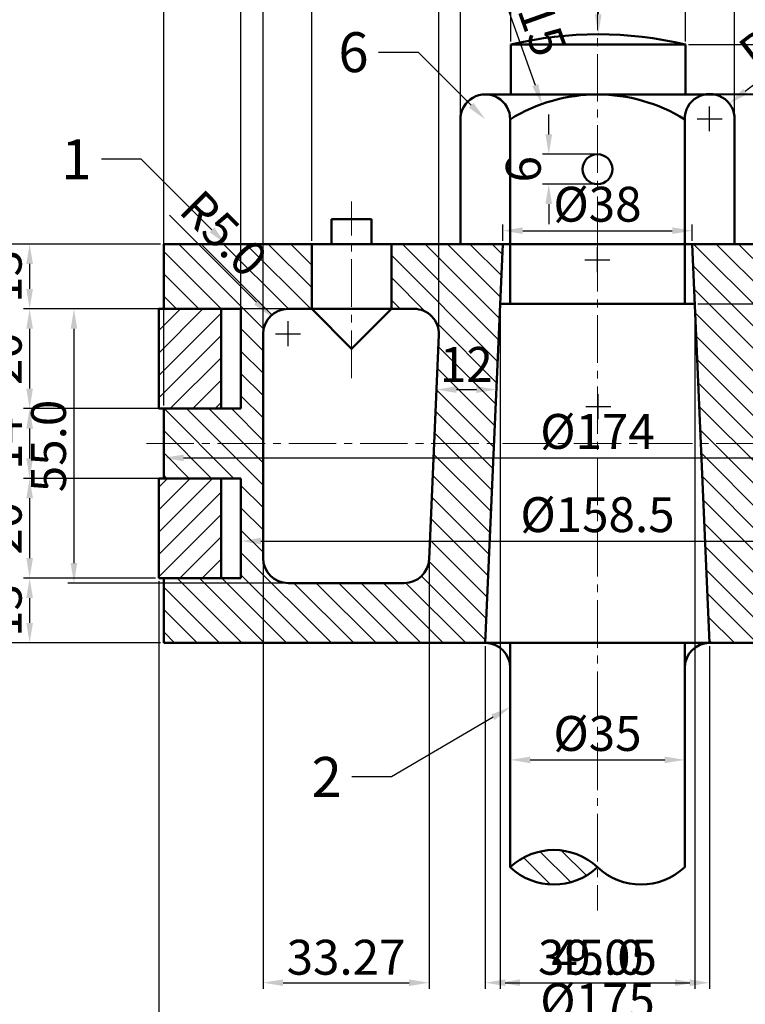
# Model space of a CAD drawing. Units: millimetres. Extents: x -21 to 693, y -570 to 295.
# Tile 4 of 7: x 107 to 253, y -4 to 193. Entities that reach past the tile are written whole.
import ezdxf
from ezdxf import colors
from ezdxf.entities.mleader import LeaderData, LeaderLine
from ezdxf.math import Vec2, Vec3

# ---------------------------------------------------------------- set-up
doc = ezdxf.new("R2010")
doc.units = ezdxf.units.MM
doc.header["$LTSCALE"] = 0.5
doc.linetypes.add('CENTER2', pattern=[28.575, 19.05, -3.175, 3.175, -3.175])
for name, color, linetype, lineweight in [('M-CNTR', 1, 'CENTER2', 18), ('M-DIMS', 2, 'Continuous', 25), ('M-HATC', 8, 'Continuous', 18), ('M-OUTL', 7, 'Continuous', 50), ('M-TEXT', 3, 'Continuous', 25)]:
    doc.layers.add(name, color=color, linetype=linetype, lineweight=lineweight)
doc.styles.get("Standard").update_dxf_attribs({"font": 'arial.ttf'})
doc.dimstyles.new('ISO-25', dxfattribs={"dimtxt": 7, "dimasz": 4, "dimexe": 1.25, "dimexo": 0.625, "dimtad": 1, "dimdec": 0, "dimtxsty": 'Standard', "dimcen": 2.5, "dimadec": 0, "dimazin": 0, "dimtfac": 1, "dimtdec": 0, "dimtofl": 0, "dimtmove": 0, "dimatfit": 3, "dimfxl": 1, "dimarcsym": 0})

# ---------------------------------------------------------------- blocks, each defined once
blk = doc.blocks.new('*U1')
at = {"layer": 'M-CNTR', "color": 0, "transparency": 16777216}
blk.add_line((0, 40), (0, -93.66), dxfattribs=at)
blk = doc.blocks.new('*U2')
at = {"layer": 'M-CNTR', "color": 0, "transparency": 16777216}
blk.add_line((90.5, 0), (-90.5, 0), dxfattribs=at)
blk = doc.blocks.new('*U3')
at = {"layer": 'M-CNTR', "color": 0, "transparency": 16777216}
blk.add_line((0, -29.38), (0, 6), dxfattribs=at)
blk = doc.blocks.new('*D5')
at = {"layer": 'Defpoints', "color": 0, "ltscale": 0.5, "transparency": 16777216}
for p in [(135.24, 81.11), (311.24, 81.11), (311.24, -8.97)]:
    blk.add_point(p, dxfattribs=at)
at = {"layer": 'M-DIMS', "color": 0, "lineweight": -2, "ltscale": 0.5, "transparency": 16777216}
for p, q in [((135.24, 80.49), (135.24, -10.22)), ((311.24, 80.49), (311.24, -10.22)), ((139.24, -8.97), (307.24, -8.97))]:
    blk.add_line(p, q, dxfattribs=at)
at = {"layer": 'M-DIMS', "color": 0, "ltscale": 0.5, "transparency": 16777216}
for points in [[(139.24, -8.31), (139.24, -9.64), (135.24, -8.97)], [(307.24, -8.31), (307.24, -9.64), (311.24, -8.97)]]:
    blk.add_solid(points, dxfattribs=at)
at = {"layer": 'M-DIMS', "color": 0, "ltscale": 0.5, "transparency": 16777216, "insert": (223.24, -4.58), "char_height": 7, "attachment_point": 5}
blk.add_mtext('%%C175', dxfattribs=at)
blk = doc.blocks.new('*D6')
at = {"layer": 'Defpoints', "color": 0, "ltscale": 0.5, "transparency": 16777216}
for p in [(136.24, 148.11), (77.7, 68.11), (136.24, 68.11)]:
    blk.add_point(p, dxfattribs=at)
at = {"layer": 'M-DIMS', "color": 0, "lineweight": -2, "ltscale": 0.5, "transparency": 16777216}
for p, q in [((135.61, 148.11), (76.45, 148.11)), ((77.7, 144.11), (77.7, 72.11)), ((135.61, 68.11), (76.45, 68.11))]:
    blk.add_line(p, q, dxfattribs=at)
at = {"layer": 'M-DIMS', "color": 0, "ltscale": 0.5, "transparency": 16777216}
for points in [[(77.04, 144.11), (78.37, 144.11), (77.7, 148.11)], [(77.04, 72.11), (78.37, 72.11), (77.7, 68.11)]]:
    blk.add_solid(points, dxfattribs=at)
at = {"layer": 'M-DIMS', "color": 0, "ltscale": 0.5, "transparency": 16777216, "insert": (73.5, 108.11), "char_height": 7, "attachment_point": 5, "rotation": 90}
blk.add_mtext('80', dxfattribs=at)
blk = doc.blocks.new('*D7')
at = {"layer": 'Defpoints', "color": 0, "ltscale": 0.5, "transparency": 16777216}
for p in [(136.24, 148.11), (109.35, 135.11), (136.24, 135.11)]:
    blk.add_point(p, dxfattribs=at)
at = {"layer": 'M-DIMS', "color": 0, "lineweight": -2, "ltscale": 0.5, "transparency": 16777216}
for p, q in [((135.61, 148.11), (108.1, 148.11)), ((109.35, 144.11), (109.35, 139.11)), ((135.61, 135.11), (108.1, 135.11))]:
    blk.add_line(p, q, dxfattribs=at)
at = {"layer": 'M-DIMS', "color": 0, "ltscale": 0.5, "transparency": 16777216}
for points in [[(108.69, 144.11), (110.02, 144.11), (109.35, 148.11)], [(108.69, 139.11), (110.02, 139.11), (109.35, 135.11)]]:
    blk.add_solid(points, dxfattribs=at)
at = {"layer": 'M-DIMS', "color": 0, "ltscale": 0.5, "transparency": 16777216, "insert": (105.15, 141.61), "char_height": 7, "attachment_point": 5, "rotation": 90}
blk.add_mtext('13', dxfattribs=at)
blk = doc.blocks.new('*D8')
at = {"layer": 'Defpoints', "color": 0, "ltscale": 0.5, "transparency": 16777216}
for p in [(135.24, 135.11), (109.35, 115.11), (136.24, 115.11)]:
    blk.add_point(p, dxfattribs=at)
at = {"layer": 'M-DIMS', "color": 0, "lineweight": -2, "ltscale": 0.5, "transparency": 16777216}
for p, q in [((134.61, 135.11), (108.1, 135.11)), ((109.35, 131.11), (109.35, 119.11)), ((135.61, 115.11), (108.1, 115.11))]:
    blk.add_line(p, q, dxfattribs=at)
at = {"layer": 'M-DIMS', "color": 0, "ltscale": 0.5, "transparency": 16777216}
for points in [[(108.69, 131.11), (110.02, 131.11), (109.35, 135.11)], [(108.69, 119.11), (110.02, 119.11), (109.35, 115.11)]]:
    blk.add_solid(points, dxfattribs=at)
at = {"layer": 'M-DIMS', "color": 0, "ltscale": 0.5, "transparency": 16777216, "insert": (105.16, 125.11), "char_height": 7, "attachment_point": 5, "rotation": 90}
blk.add_mtext('20', dxfattribs=at)
blk = doc.blocks.new('*D9')
at = {"layer": 'Defpoints', "color": 0, "ltscale": 0.5, "transparency": 16777216}
for p in [(136.24, 115.11), (109.35, 101.11), (136.24, 101.11)]:
    blk.add_point(p, dxfattribs=at)
at = {"layer": 'M-DIMS', "color": 0, "lineweight": -2, "ltscale": 0.5, "transparency": 16777216}
for p, q in [((135.61, 115.11), (108.1, 115.11)), ((109.35, 111.11), (109.35, 105.11)), ((135.61, 101.11), (108.1, 101.11))]:
    blk.add_line(p, q, dxfattribs=at)
at = {"layer": 'M-DIMS', "color": 0, "ltscale": 0.5, "transparency": 16777216}
for points in [[(108.69, 111.11), (110.02, 111.11), (109.35, 115.11)], [(108.69, 105.11), (110.02, 105.11), (109.35, 101.11)]]:
    blk.add_solid(points, dxfattribs=at)
at = {"layer": 'M-DIMS', "color": 0, "ltscale": 0.5, "transparency": 16777216, "insert": (105.21, 108.11), "char_height": 7, "attachment_point": 5, "rotation": 90}
blk.add_mtext('14', dxfattribs=at)
blk = doc.blocks.new('*D10')
at = {"layer": 'Defpoints', "color": 0, "ltscale": 0.5, "transparency": 16777216}
for p in [(136.24, 101.11), (109.35, 81.11), (135.24, 81.11)]:
    blk.add_point(p, dxfattribs=at)
at = {"layer": 'M-DIMS', "color": 0, "lineweight": -2, "ltscale": 0.5, "transparency": 16777216}
for p, q in [((135.61, 101.11), (108.1, 101.11)), ((109.35, 97.11), (109.35, 85.11)), ((134.61, 81.11), (108.1, 81.11))]:
    blk.add_line(p, q, dxfattribs=at)
at = {"layer": 'M-DIMS', "color": 0, "ltscale": 0.5, "transparency": 16777216}
for points in [[(108.69, 97.11), (110.02, 97.11), (109.35, 101.11)], [(108.69, 85.11), (110.02, 85.11), (109.35, 81.11)]]:
    blk.add_solid(points, dxfattribs=at)
at = {"layer": 'M-DIMS', "color": 0, "ltscale": 0.5, "transparency": 16777216, "insert": (105.16, 91.11), "char_height": 7, "attachment_point": 5, "rotation": 90}
blk.add_mtext('20', dxfattribs=at)
blk = doc.blocks.new('*D11')
at = {"layer": 'Defpoints', "color": 0, "ltscale": 0.5, "transparency": 16777216}
for p in [(129.36, 81.11), (109.35, 68.11), (136.24, 68.11)]:
    blk.add_point(p, dxfattribs=at)
at = {"layer": 'M-DIMS', "color": 0, "lineweight": -2, "ltscale": 0.5, "transparency": 16777216}
for p, q in [((128.74, 81.11), (108.1, 81.11)), ((109.35, 77.11), (109.35, 72.11)), ((135.61, 68.11), (108.1, 68.11))]:
    blk.add_line(p, q, dxfattribs=at)
at = {"layer": 'M-DIMS', "color": 0, "ltscale": 0.5, "transparency": 16777216}
for points in [[(108.69, 77.11), (110.02, 77.11), (109.35, 81.11)], [(108.69, 72.11), (110.02, 72.11), (109.35, 68.11)]]:
    blk.add_solid(points, dxfattribs=at)
at = {"layer": 'M-DIMS', "color": 0, "ltscale": 0.5, "transparency": 16777216, "insert": (105.15, 74.61), "char_height": 7, "attachment_point": 5, "rotation": 90}
blk.add_mtext('13', dxfattribs=at)
blk = doc.blocks.new('*D12')
at = {"layer": 'Defpoints', "color": 0, "ltscale": 0.5, "transparency": 16777216}
for p in [(190.95, 118.92), (202.96, 118.92), (202.96, 118.92)]:
    blk.add_point(p, dxfattribs=at)
at = {"layer": 'M-DIMS', "color": 0, "lineweight": -2, "ltscale": 0.5, "transparency": 16777216}
for p, q in [((190.95, 119.54), (190.95, 120.17)), ((194.95, 118.92), (198.96, 118.92)), ((202.96, 119.54), (202.96, 120.17))]:
    blk.add_line(p, q, dxfattribs=at)
at = {"layer": 'M-DIMS', "color": 0, "ltscale": 0.5, "transparency": 16777216}
for points in [[(194.95, 119.59), (194.95, 118.25), (190.95, 118.92)], [(198.96, 119.59), (198.96, 118.25), (202.96, 118.92)]]:
    blk.add_solid(points, dxfattribs=at)
at = {"layer": 'M-DIMS', "color": 0, "ltscale": 0.5, "transparency": 16777216, "insert": (196.95, 123.06), "char_height": 7, "attachment_point": 5}
blk.add_mtext('12', dxfattribs=at)
blk = doc.blocks.new('*D13')
at = {"layer": 'Defpoints', "color": 0, "ltscale": 0.5, "transparency": 16777216}
for p in [(151.74, 91.11), (294.74, 91.11), (294.74, 88.53)]:
    blk.add_point(p, dxfattribs=at)
at = {"layer": 'M-DIMS', "color": 0, "lineweight": -2, "ltscale": 0.5, "transparency": 16777216}
for p, q in [((151.74, 90.49), (151.74, 87.28)), ((294.74, 90.49), (294.74, 87.28)), ((155.74, 88.53), (290.74, 88.53))]:
    blk.add_line(p, q, dxfattribs=at)
at = {"layer": 'M-DIMS', "color": 0, "ltscale": 0.5, "transparency": 16777216}
for points in [[(155.74, 89.2), (155.74, 87.87), (151.74, 88.53)], [(290.74, 89.2), (290.74, 87.87), (294.74, 88.53)]]:
    blk.add_solid(points, dxfattribs=at)
at = {"layer": 'M-DIMS', "color": 0, "ltscale": 0.5, "transparency": 16777216, "insert": (223.24, 92.93), "char_height": 7, "attachment_point": 5}
blk.add_mtext('%%C158.5', dxfattribs=at)
blk = doc.blocks.new('*D14')
at = {"layer": 'Defpoints', "color": 0, "ltscale": 0.5, "transparency": 16777216}
for p in [(136.24, 108.11), (310.24, 108.11), (310.24, 105.22)]:
    blk.add_point(p, dxfattribs=at)
at = {"layer": 'M-DIMS', "color": 0, "lineweight": -2, "ltscale": 0.5, "transparency": 16777216}
for p, q in [((136.24, 107.49), (136.24, 103.97)), ((310.24, 107.49), (310.24, 103.97)), ((140.24, 105.22), (306.24, 105.22))]:
    blk.add_line(p, q, dxfattribs=at)
at = {"layer": 'M-DIMS', "color": 0, "ltscale": 0.5, "transparency": 16777216}
for points in [[(140.24, 105.89), (140.24, 104.55), (136.24, 105.22)], [(306.24, 105.89), (306.24, 104.55), (310.24, 105.22)]]:
    blk.add_solid(points, dxfattribs=at)
at = {"layer": 'M-DIMS', "color": 0, "ltscale": 0.5, "transparency": 16777216, "insert": (223.24, 109.62), "char_height": 7, "attachment_point": 5}
blk.add_mtext('%%C174', dxfattribs=at)
blk = doc.blocks.new('*D15')
at = {"layer": 'Defpoints', "color": 0, "ltscale": 0.5, "transparency": 16777216}
for p in [(242.24, 150.79), (204.24, 148.11), (242.24, 148.11)]:
    blk.add_point(p, dxfattribs=at)
at = {"layer": 'M-DIMS', "color": 0, "lineweight": -2, "ltscale": 0.5, "transparency": 16777216}
for p, q in [((204.24, 148.74), (204.24, 152.04)), ((208.24, 150.79), (238.24, 150.79)), ((242.24, 148.74), (242.24, 152.04))]:
    blk.add_line(p, q, dxfattribs=at)
at = {"layer": 'M-DIMS', "color": 0, "ltscale": 0.5, "transparency": 16777216}
for points in [[(208.24, 151.46), (208.24, 150.13), (204.24, 150.79)], [(238.24, 151.46), (238.24, 150.13), (242.24, 150.79)]]:
    blk.add_solid(points, dxfattribs=at)
at = {"layer": 'M-DIMS', "color": 0, "ltscale": 0.5, "transparency": 16777216, "insert": (223.24, 155.19), "char_height": 7, "attachment_point": 5}
blk.add_mtext('%%C38', dxfattribs=at)
blk = doc.blocks.new('*D16')
at = {"layer": 'Defpoints', "color": 0, "ltscale": 0.5, "transparency": 16777216}
for p in [(223.24, 166.11), (213.47, 160.11), (223.24, 160.11)]:
    blk.add_point(p, dxfattribs=at)
at = {"layer": 'M-DIMS', "color": 0, "lineweight": -2, "ltscale": 0.5, "transparency": 16777216}
for p, q in [((213.47, 170.11), (213.47, 174.11)), ((222.61, 166.11), (212.22, 166.11)), ((222.61, 160.11), (212.22, 160.11)), ((213.47, 156.11), (213.47, 152.11))]:
    blk.add_line(p, q, dxfattribs=at)
at = {"layer": 'M-DIMS', "color": 0, "ltscale": 0.5, "transparency": 16777216}
for points in [[(212.8, 170.11), (214.14, 170.11), (213.47, 166.11)], [(212.8, 156.11), (214.14, 156.11), (213.47, 160.11)]]:
    blk.add_solid(points, dxfattribs=at)
at = {"layer": 'M-DIMS', "color": 0, "ltscale": 0.5, "transparency": 16777216, "insert": (209.27, 163.11), "char_height": 7, "attachment_point": 5, "rotation": 90}
blk.add_mtext('6', dxfattribs=at)
blk = doc.blocks.new('*D17')
at = {"layer": 'Defpoints', "color": 0, "ltscale": 0.5, "transparency": 16777216}
for p in [(205.74, 45.61), (240.74, 45.61), (240.74, 44.65)]:
    blk.add_point(p, dxfattribs=at)
at = {"layer": 'M-DIMS', "color": 0, "lineweight": -2, "ltscale": 0.5, "transparency": 16777216}
for p, q in [((205.74, 44.99), (205.74, 43.4)), ((209.74, 44.65), (236.74, 44.65)), ((240.74, 44.99), (240.74, 43.4))]:
    blk.add_line(p, q, dxfattribs=at)
at = {"layer": 'M-DIMS', "color": 0, "ltscale": 0.5, "transparency": 16777216}
for points in [[(209.74, 45.31), (209.74, 43.98), (205.74, 44.65)], [(236.74, 45.31), (236.74, 43.98), (240.74, 44.65)]]:
    blk.add_solid(points, dxfattribs=at)
at = {"layer": 'M-DIMS', "color": 0, "ltscale": 0.5, "transparency": 16777216, "insert": (223.24, 49.04), "char_height": 7, "attachment_point": 5}
blk.add_mtext('%%C35', dxfattribs=at)
blk = doc.blocks.new('SCREW-PLUG')
for p, q in [((4, 21), (4, 26)), ((4, 26), (12, 26)), ((12, 26), (12, 21)), ((0, 21), (0, 8)), ((16, 21), (16, 8)), ((0, 8), (8, 0)), ((16, 8), (8, 0))]:
    blk.add_line(p, q)
blk = doc.blocks.new('*D49')
at = {"layer": 'Defpoints', "color": 0, "ltscale": 0.5, "transparency": 16777216}
for p in [(191.43, 210.86), (156.19, 130.11), (191.43, 129.89)]:
    blk.add_point(p, dxfattribs=at)
at = {"layer": 'M-DIMS', "color": 0, "lineweight": -2, "ltscale": 0.5, "transparency": 16777216}
for p, q in [((156.19, 130.74), (156.19, 212.11)), ((191.43, 130.52), (191.43, 212.11)), ((160.19, 210.86), (187.43, 210.86))]:
    blk.add_line(p, q, dxfattribs=at)
at = {"layer": 'M-DIMS', "color": 0, "ltscale": 0.5, "transparency": 16777216}
for points in [[(160.19, 211.53), (160.19, 210.2), (156.19, 210.86)], [(187.43, 211.53), (187.43, 210.2), (191.43, 210.86)]]:
    blk.add_solid(points, dxfattribs=at)
at = {"layer": 'M-DIMS', "color": 0, "ltscale": 0.5, "transparency": 16777216, "insert": (173.81, 215.07), "char_height": 7, "attachment_point": 5}
blk.add_mtext('35.24', dxfattribs=at)
blk = doc.blocks.new('*D50')
at = {"layer": 'Defpoints', "color": 0, "ltscale": 0.5, "transparency": 16777216}
for p in [(156.19, 85.11), (189.46, 84.89), (189.46, -0.04)]:
    blk.add_point(p, dxfattribs=at)
at = {"layer": 'M-DIMS', "color": 0, "lineweight": -2, "ltscale": 0.5, "transparency": 16777216}
for p, q in [((156.19, 84.49), (156.19, -1.29)), ((189.46, 84.27), (189.46, -1.29)), ((160.19, -0.04), (185.46, -0.04))]:
    blk.add_line(p, q, dxfattribs=at)
at = {"layer": 'M-DIMS', "color": 0, "ltscale": 0.5, "transparency": 16777216}
for points in [[(160.19, 0.62), (160.19, -0.71), (156.19, -0.04)], [(185.46, 0.62), (185.46, -0.71), (189.46, -0.04)]]:
    blk.add_solid(points, dxfattribs=at)
at = {"layer": 'M-DIMS', "color": 0, "ltscale": 0.5, "transparency": 16777216, "insert": (172.82, 4.16), "char_height": 7, "attachment_point": 5}
blk.add_mtext('33.27', dxfattribs=at)
blk = doc.blocks.new('*D51')
at = {"layer": 'Defpoints', "color": 0, "ltscale": 0.5, "transparency": 16777216}
for p in [(161.19, 135.11), (118.24, 80.11), (161.19, 80.11)]:
    blk.add_point(p, dxfattribs=at)
at = {"layer": 'M-DIMS', "color": 0, "lineweight": -2, "ltscale": 0.5, "transparency": 16777216}
for p, q in [((160.56, 135.11), (116.99, 135.11)), ((118.24, 131.11), (118.24, 84.11)), ((160.56, 80.11), (116.99, 80.11))]:
    blk.add_line(p, q, dxfattribs=at)
at = {"layer": 'M-DIMS', "color": 0, "ltscale": 0.5, "transparency": 16777216}
for points in [[(117.57, 131.11), (118.9, 131.11), (118.24, 135.11)], [(117.57, 84.11), (118.9, 84.11), (118.24, 80.11)]]:
    blk.add_solid(points, dxfattribs=at)
at = {"layer": 'M-DIMS', "color": 0, "ltscale": 0.5, "transparency": 16777216, "insert": (114.04, 107.61), "char_height": 7, "attachment_point": 5, "rotation": 90}
blk.add_mtext('55.0', dxfattribs=at)
blk = doc.blocks.new('*D52')
at = {"layer": 'Defpoints', "color": 0, "ltscale": 0.5, "transparency": 16777216}
for p in [(151.74, 210.86), (136.24, 115.11), (151.74, 115.11)]:
    blk.add_point(p, dxfattribs=at)
at = {"layer": 'M-DIMS', "color": 0, "lineweight": -2, "ltscale": 0.5, "transparency": 16777216}
for p, q in [((136.24, 115.74), (136.24, 212.11)), ((151.74, 115.74), (151.74, 212.11)), ((140.24, 210.86), (147.74, 210.86)), ((151.74, 210.86), (174.56, 210.86))]:
    blk.add_line(p, q, dxfattribs=at)
at = {"layer": 'M-DIMS', "color": 0, "ltscale": 0.5, "transparency": 16777216}
for points in [[(140.24, 211.53), (140.24, 210.2), (136.24, 210.86)], [(147.74, 211.53), (147.74, 210.2), (151.74, 210.86)]]:
    blk.add_solid(points, dxfattribs=at)
at = {"layer": 'M-DIMS', "color": 0, "ltscale": 0.5, "transparency": 16777216, "insert": (165.15, 215.06), "char_height": 7, "attachment_point": 5}
blk.add_mtext('15.5', dxfattribs=at)
blk = doc.blocks.new('*D53')
at = {"layer": 'Defpoints', "color": 0, "ltscale": 0.5, "transparency": 16777216}
for p in [(203.71, 136.11), (242.76, 136.11), (242.76, -0.04)]:
    blk.add_point(p, dxfattribs=at)
at = {"layer": 'M-DIMS', "color": 0, "lineweight": -2, "ltscale": 0.5, "transparency": 16777216}
for p, q in [((203.71, 135.49), (203.71, -1.29)), ((242.76, 135.49), (242.76, -1.29)), ((207.71, -0.04), (238.76, -0.04))]:
    blk.add_line(p, q, dxfattribs=at)
at = {"layer": 'M-DIMS', "color": 0, "ltscale": 0.5, "transparency": 16777216}
for points in [[(207.71, 0.62), (207.71, -0.71), (203.71, -0.04)], [(238.76, 0.62), (238.76, -0.71), (242.76, -0.04)]]:
    blk.add_solid(points, dxfattribs=at)
at = {"layer": 'M-DIMS', "color": 0, "ltscale": 0.5, "transparency": 16777216, "insert": (223.24, 4.16), "char_height": 7, "attachment_point": 5}
blk.add_mtext('39.05', dxfattribs=at)
blk = doc.blocks.new('*D54')
at = {"layer": 'Defpoints', "color": 0, "ltscale": 0.5, "transparency": 16777216}
for p in [(200.74, 68.11), (245.74, 68.11), (245.74, -0.04)]:
    blk.add_point(p, dxfattribs=at)
at = {"layer": 'M-DIMS', "color": 0, "lineweight": -2, "ltscale": 0.5, "transparency": 16777216}
for p, q in [((200.74, 67.49), (200.74, -1.29)), ((245.74, 67.49), (245.74, -1.29)), ((204.74, -0.04), (241.74, -0.04))]:
    blk.add_line(p, q, dxfattribs=at)
at = {"layer": 'M-DIMS', "color": 0, "ltscale": 0.5, "transparency": 16777216}
for points in [[(204.74, 0.62), (204.74, -0.71), (200.74, -0.04)], [(241.74, 0.62), (241.74, -0.71), (245.74, -0.04)]]:
    blk.add_solid(points, dxfattribs=at)
at = {"layer": 'M-DIMS', "color": 0, "ltscale": 0.5, "transparency": 16777216, "insert": (223.24, 4.16), "char_height": 7, "attachment_point": 5}
blk.add_mtext('45.0', dxfattribs=at)
blk = doc.blocks.new('*D55')
at = {"layer": 'Defpoints', "color": 0, "ltscale": 0.5, "transparency": 16777216}
for p in [(242.24, 148.11), (242.76, 136.11), (328.24, 136.11)]:
    blk.add_point(p, dxfattribs=at)
at = {"layer": 'M-DIMS', "color": 0, "lineweight": -2, "ltscale": 0.5, "transparency": 16777216}
for p, q in [((242.86, 148.11), (329.49, 148.11)), ((328.24, 144.11), (328.24, 140.11)), ((243.39, 136.11), (329.49, 136.11)), ((328.24, 136.11), (328.24, 113.36))]:
    blk.add_line(p, q, dxfattribs=at)
at = {"layer": 'M-DIMS', "color": 0, "ltscale": 0.5, "transparency": 16777216}
for points in [[(327.57, 144.11), (328.9, 144.11), (328.24, 148.11)], [(327.57, 140.11), (328.9, 140.11), (328.24, 136.11)]]:
    blk.add_solid(points, dxfattribs=at)
at = {"layer": 'M-DIMS', "color": 0, "ltscale": 0.5, "transparency": 16777216, "insert": (324.04, 122.74), "char_height": 7, "attachment_point": 5, "rotation": 90}
blk.add_mtext('12.0', dxfattribs=at)
blk = doc.blocks.new('*D56')
at = {"layer": 'Defpoints', "color": 0, "ltscale": 0.5, "transparency": 16777216}
for p in [(165.92, 210.86), (136.24, 148.11), (165.92, 148.11)]:
    blk.add_point(p, dxfattribs=at)
at = {"layer": 'M-DIMS', "color": 0, "lineweight": -2, "ltscale": 0.5, "transparency": 16777216}
for p, q in [((136.24, 148.74), (136.24, 212.11)), ((165.92, 148.74), (165.92, 212.11)), ((140.24, 210.86), (161.92, 210.86)), ((165.92, 210.86), (200.4, 210.86))]:
    blk.add_line(p, q, dxfattribs=at)
at = {"layer": 'M-DIMS', "color": 0, "ltscale": 0.5, "transparency": 16777216}
for points in [[(140.24, 211.53), (140.24, 210.2), (136.24, 210.86)], [(161.92, 211.53), (161.92, 210.2), (165.92, 210.86)]]:
    blk.add_solid(points, dxfattribs=at)
at = {"layer": 'M-DIMS', "color": 0, "ltscale": 0.5, "transparency": 16777216, "insert": (185.16, 215.06), "char_height": 7, "attachment_point": 5}
blk.add_mtext('29.685', dxfattribs=at)
blk = doc.blocks.new('*D61')
at = {"layer": 'Defpoints', "color": 0, "ltscale": 0.5, "transparency": 16777216}
for p in [(250.74, 210.86), (195.74, 173.12), (250.74, 173.32)]:
    blk.add_point(p, dxfattribs=at)
at = {"layer": 'M-DIMS', "color": 0, "lineweight": -2, "ltscale": 0.5, "transparency": 16777216}
for p, q in [((195.74, 173.75), (195.74, 212.11)), ((250.74, 173.95), (250.74, 212.11)), ((199.74, 210.86), (246.74, 210.86))]:
    blk.add_line(p, q, dxfattribs=at)
at = {"layer": 'M-DIMS', "color": 0, "ltscale": 0.5, "transparency": 16777216}
for points in [[(199.74, 211.53), (199.74, 210.2), (195.74, 210.86)], [(246.74, 211.53), (246.74, 210.2), (250.74, 210.86)]]:
    blk.add_solid(points, dxfattribs=at)
at = {"layer": 'M-DIMS', "color": 0, "ltscale": 0.5, "transparency": 16777216, "insert": (223.24, 215.06), "char_height": 7, "attachment_point": 5}
blk.add_mtext('55.0', dxfattribs=at)
blk = doc.blocks.new('*D62')
at = {"layer": 'Defpoints', "color": 0, "ltscale": 0.5, "transparency": 16777216}
for p in [(245.74, 178.22), (328.24, 178.22), (250.74, 148.11)]:
    blk.add_point(p, dxfattribs=at)
at = {"layer": 'M-DIMS', "color": 0, "lineweight": -2, "ltscale": 0.5, "transparency": 16777216}
for p, q in [((328.24, 178.22), (328.24, 212.58)), ((246.36, 178.22), (329.49, 178.22)), ((328.24, 152.11), (328.24, 174.22)), ((251.36, 148.11), (329.49, 148.11))]:
    blk.add_line(p, q, dxfattribs=at)
at = {"layer": 'M-DIMS', "color": 0, "ltscale": 0.5, "transparency": 16777216}
for points in [[(327.57, 174.22), (328.9, 174.22), (328.24, 178.22)], [(327.57, 152.11), (328.9, 152.11), (328.24, 148.11)]]:
    blk.add_solid(points, dxfattribs=at)
at = {"layer": 'M-DIMS', "color": 0, "ltscale": 0.5, "transparency": 16777216, "insert": (324.04, 197.4), "char_height": 7, "attachment_point": 5, "rotation": 90}
blk.add_mtext('30.105', dxfattribs=at)
blk = doc.blocks.new('*D63')
at = {"layer": 'Defpoints', "color": 0, "ltscale": 0.5, "transparency": 16777216}
for p in [(240.89, 210.86), (205.89, 188.11), (240.89, 188.11)]:
    blk.add_point(p, dxfattribs=at)
at = {"layer": 'M-DIMS', "color": 0, "lineweight": -2, "ltscale": 0.5, "transparency": 16777216}
for p, q in [((205.89, 188.74), (205.89, 212.11)), ((240.89, 188.74), (240.89, 212.11)), ((209.89, 210.86), (236.89, 210.86))]:
    blk.add_line(p, q, dxfattribs=at)
at = {"layer": 'M-DIMS', "color": 0, "ltscale": 0.5, "transparency": 16777216}
for points in [[(209.89, 211.53), (209.89, 210.2), (205.89, 210.86)], [(236.89, 211.53), (236.89, 210.2), (240.89, 210.86)]]:
    blk.add_solid(points, dxfattribs=at)
at = {"layer": 'M-DIMS', "color": 0, "ltscale": 0.5, "transparency": 16777216, "insert": (223.39, 215.07), "char_height": 7, "attachment_point": 5}
blk.add_mtext('35.0', dxfattribs=at)
blk = doc.blocks.new('*D64')
at = {"layer": 'Defpoints', "color": 0, "ltscale": 0.5, "transparency": 16777216}
for p in [(240.89, 188.11), (328.24, 188.11), (240.89, 178.11)]:
    blk.add_point(p, dxfattribs=at)
at = {"layer": 'M-DIMS', "color": 0, "lineweight": -2, "ltscale": 0.5, "transparency": 16777216}
for p, q in [((328.24, 188.11), (328.24, 210.86)), ((241.51, 188.11), (329.49, 188.11)), ((328.24, 182.11), (328.24, 184.11)), ((241.51, 178.11), (329.49, 178.11))]:
    blk.add_line(p, q, dxfattribs=at)
at = {"layer": 'M-DIMS', "color": 0, "ltscale": 0.5, "transparency": 16777216}
for points in [[(327.57, 184.11), (328.9, 184.11), (328.24, 188.11)], [(327.57, 182.11), (328.9, 182.11), (328.24, 178.11)]]:
    blk.add_solid(points, dxfattribs=at)
at = {"layer": 'M-DIMS', "color": 0, "ltscale": 0.5, "transparency": 16777216, "insert": (324.04, 201.49), "char_height": 7, "attachment_point": 5, "rotation": 90}
blk.add_mtext('10.0', dxfattribs=at)
blk = doc.blocks.new('*D68')
at = {"layer": 'Defpoints', "color": 0, "ltscale": 0.5, "transparency": 16777216}
for p in [(157.65, 133.65), (161.19, 130.11)]:
    blk.add_point(p, dxfattribs=at)
at = {"layer": 'M-DIMS', "color": 0, "lineweight": -2, "ltscale": 0.5, "transparency": 16777216}
for p, q in [((137.38, 153.92), (154.82, 136.48)), ((161.19, 127.61), (161.19, 132.61)), ((158.69, 130.11), (163.69, 130.11))]:
    blk.add_line(p, q, dxfattribs=at)
at = {"layer": 'M-DIMS', "color": 0, "ltscale": 0.5, "transparency": 16777216}
blk.add_solid([(155.29, 136.95), (154.35, 136.01), (157.65, 133.65)], dxfattribs=at)
at = {"layer": 'M-DIMS', "color": 0, "ltscale": 0.5, "transparency": 16777216, "insert": (147.66, 149.58), "char_height": 7, "attachment_point": 5, "rotation": 314.9981}
blk.add_mtext('R5.0', dxfattribs=at)
blk = doc.blocks.new('*D69')
at = {"layer": 'Defpoints', "color": 0, "ltscale": 0.5, "transparency": 16777216}
for p in [(249.7, 176.27), (245.74, 173.22)]:
    blk.add_point(p, dxfattribs=at)
at = {"layer": 'M-DIMS', "color": 0, "lineweight": -2, "ltscale": 0.5, "transparency": 16777216}
for p, q in [((279.98, 199.59), (252.87, 178.71)), ((245.74, 170.72), (245.74, 175.72)), ((243.24, 173.22), (248.24, 173.22))]:
    blk.add_line(p, q, dxfattribs=at)
at = {"layer": 'M-DIMS', "color": 0, "ltscale": 0.5, "transparency": 16777216}
blk.add_solid([(252.46, 179.24), (253.28, 178.18), (249.7, 176.27)], dxfattribs=at)
at = {"layer": 'M-DIMS', "color": 0, "ltscale": 0.5, "transparency": 16777216, "insert": (265.45, 193.7), "char_height": 7, "attachment_point": 5, "rotation": 37.6005}
blk.add_mtext('R5.001', dxfattribs=at)
blk = doc.blocks.new('*D70')
at = {"layer": 'Defpoints', "color": 0, "ltscale": 0.5, "transparency": 16777216}
for p in [(212.11, 176.19), (223.23, 144.96)]:
    blk.add_point(p, dxfattribs=at)
at = {"layer": 'M-DIMS', "color": 0, "lineweight": -2, "ltscale": 0.5, "transparency": 16777216}
for p, q in [((198.82, 213.52), (210.77, 179.96)), ((223.23, 142.46), (223.23, 147.46)), ((220.73, 144.96), (225.73, 144.96))]:
    blk.add_line(p, q, dxfattribs=at)
at = {"layer": 'M-DIMS', "color": 0, "ltscale": 0.5, "transparency": 16777216}
blk.add_solid([(211.4, 180.18), (210.14, 179.74), (212.11, 176.19)], dxfattribs=at)
at = {"layer": 'M-DIMS', "color": 0, "ltscale": 0.5, "transparency": 16777216, "insert": (208.08, 200.03), "char_height": 7, "attachment_point": 5, "rotation": 289.5972}
blk.add_mtext('R33.15', dxfattribs=at)
blk = doc.blocks.new('*D71')
at = {"layer": 'Defpoints', "color": 0, "ltscale": 0.5, "transparency": 16777216}
for p in [(223.39, 190.19), (223.39, 115.5)]:
    blk.add_point(p, dxfattribs=at)
at = {"layer": 'M-DIMS', "color": 0, "lineweight": -2, "ltscale": 0.5, "transparency": 16777216}
for p, q in [((223.39, 250.8), (223.39, 194.19)), ((223.39, 113), (223.39, 118)), ((220.89, 115.5), (225.89, 115.5))]:
    blk.add_line(p, q, dxfattribs=at)
at = {"layer": 'M-DIMS', "color": 0, "ltscale": 0.5, "transparency": 16777216}
blk.add_solid([(222.72, 194.19), (224.06, 194.19), (223.39, 190.19)], dxfattribs=at)
at = {"layer": 'M-DIMS', "color": 0, "ltscale": 0.5, "transparency": 16777216, "insert": (219.19, 235.01), "char_height": 7, "attachment_point": 5, "rotation": 89.9979}
blk.add_mtext('R74.69', dxfattribs=at)

msp = doc.modelspace()

# ---------------------------------------------------------------- hatches: boundary and pattern name
at = {"layer": 'M-HATC'}
h = msp.add_hatch(dxfattribs=at)
h.set_pattern_fill('ANSI31', color=256, angle=90)
h.paths.add_polyline_path([(136.2368, 148.1134), (136.2368, 135.1134), (151.7368, 135.1134), (151.7368, 115.1134), (136.2368, 115.1134), (136.2368, 108.1134), (156.1864, 108.1134), (156.1864, 130.1134, -0.41421356), (161.1864, 135.1134), (165.9215, 135.1134), (165.9215, 148.1134)])
h.paths.add_polyline_path([(151.7368, 101.1134), (151.7368, 81.1134), (136.2368, 81.1134), (136.2368, 68.1134), (200.7368, 68.1134), (202.4868, 108.1134), (190.4753, 108.1134), (189.4595, 84.8948, -0.40146486), (184.4643, 80.1134), (161.1864, 80.1134, -0.41421356), (156.1864, 85.1134), (156.1864, 108.1134), (136.2368, 108.1134), (136.2368, 101.1134)])
h.paths.add_polyline_path([(204.2368, 148.1134), (195.7368, 148.1134), (181.9215, 148.1134), (181.9215, 135.1134), (186.4331, 135.1134, -0.42707823), (191.4283, 129.8948), (190.4753, 108.1134), (202.4868, 108.1134)])
h.paths.add_polyline_path([(310.2368, 68.1134), (310.2368, 81.1134), (294.7368, 81.1134), (294.7368, 101.1134), (310.2368, 101.1134), (310.2368, 108.1134), (290.2872, 108.1134), (290.2872, 85.1134, -0.41421356), (285.2872, 80.1134), (262.0093, 80.1134, -0.40146486), (257.0141, 84.8948), (255.9983, 108.1134), (243.9868, 108.1134), (245.7368, 68.1134)])
h.paths.add_polyline_path([(243.9868, 108.1134), (255.9983, 108.1134), (255.0454, 129.8948, -0.42707823), (260.0406, 135.1134), (264.5522, 135.1134), (264.5522, 148.1134), (242.2368, 148.1134)])
h.paths.add_polyline_path([(280.5522, 135.1134), (285.2872, 135.1134, -0.41421356), (290.2872, 130.1134), (290.2872, 108.1134), (310.2368, 108.1134), (310.2368, 115.1134), (294.7368, 115.1134), (294.7368, 135.1134), (310.2368, 135.1134), (310.2368, 148.1134), (280.5522, 148.1134)])
h = msp.add_hatch(dxfattribs=at)
h.set_pattern_fill('ANSI31', color=256)
h.paths.add_polyline_path([(147.7368, 135.1134), (135.2368, 135.1134), (135.2368, 115.1134), (147.7368, 115.1134)])
h.paths.add_polyline_path([(147.7368, 101.1134), (135.2368, 101.1134), (135.2368, 81.1134), (147.7368, 81.1134)])
at = {"layer": 'M-HATC', "ltscale": 0.5}
h = msp.add_hatch(dxfattribs=at)
h.set_pattern_fill('ANSI31', color=256, angle=90)
h.paths.add_polyline_path([(205.7368, 23.1134, 0.39671485), (223.2368, 23.1134, 0.39671485)])

# ---------------------------------------------------------------- linework, layer by layer
at = {"layer": 'M-CNTR'}
msp.add_line((223.2368, 148.1134), (223.2368, 196.364), dxfattribs=at)
at = {"layer": 'M-OUTL'}
for p, q in [((205.8872, 178.1134), (205.8872, 188.1134)), ((205.8872, 188.1134), (240.8872, 188.1134)), ((240.8872, 188.1134), (240.8872, 178.1134)), ((246.7541, 178.1134), (200.5149, 178.1134)), ((195.7368, 173.1232), (195.7368, 148.1134)), ((205.7368, 173.1232), (205.7368, 136.1134)), ((240.7368, 136.1134), (240.7368, 173.3203)), ((250.7368, 148.1134), (250.7368, 173.3203)), ((136.2368, 148.1134), (136.2368, 135.1134)), ((310.2368, 148.1134), (136.2368, 148.1134)), ((195.7368, 148.1134), (250.7368, 148.1134)), ((200.7368, 68.1134), (204.2368, 148.1134)), ((245.7368, 68.1134), (242.2368, 148.1134)), ((151.7368, 135.1134), (135.2368, 135.1134)), ((135.2368, 135.1134), (135.2368, 115.1134)), ((147.7368, 115.1134), (147.7368, 135.1134)), ((151.7368, 115.1134), (151.7368, 135.1134)), ((161.1864, 135.1134), (186.4331, 135.1134)), ((203.7118, 136.1134), (242.7618, 136.1134)), ((156.1864, 130.1134), (156.1864, 85.1134)), ((189.4595, 84.8948), (191.4283, 129.8948)), ((135.2368, 115.1134), (151.7368, 115.1134)), ((136.2368, 115.1134), (136.2368, 101.1134)), ((151.7368, 101.1134), (135.2368, 101.1134)), ((135.2368, 101.1134), (135.2368, 81.1134)), ((147.7368, 81.1134), (147.7368, 101.1134)), ((151.7368, 81.1134), (151.7368, 101.1134)), ((135.2368, 81.1134), (151.7368, 81.1134)), ((136.2368, 81.1134), (136.2368, 68.1134)), ((161.1864, 80.1134), (184.4643, 80.1134)), ((136.2368, 68.1134), (310.2368, 68.1134)), ((205.7368, 23.1134), (205.7368, 68.1134)), ((240.7368, 68.1134), (240.7368, 23.1134))]:
    msp.add_line(p, q, dxfattribs=at)
msp.add_circle((223.2368, 163.1134), 3, dxfattribs=at)
for centre, radius, start, end in [((223.3872, 115.5045), 74.688, 76.449165, 103.550835), ((200.7368, 173.1183), 5, 359.943578, 180.056422), ((223.2289, 144.9606), 33.1527, 58.1229, 121.844859), ((245.7368, 173.2169), 5.0011, 358.814236, 181.185764), ((161.1864, 130.1134), 5, 90, 180), ((186.4331, 130.1134), 5, 357.494907, 90), ((161.1864, 85.1134), 5, 180, 270), ((184.4643, 85.1134), 5, 270, 357.494907), ((200.7368, 63.1134), 5, 0, 90), ((245.7368, 63.1134), 5, 90, 180), ((214.4868, 13.8209), 12.7637, 46.722074, 133.277926), ((214.4868, 32.4058), 12.7637, 226.722074, 313.277926), ((231.9868, 32.4058), 12.7637, 226.722074, 313.277926)]:
    msp.add_arc(centre, radius, start, end, dxfattribs=at)

# ---------------------------------------------------------------- block references
at = {"layer": 'M-CNTR'}
for name, p in [('*U3', (173.9215, 150.6134)), ('*U1', (223.2368, 108.1134)), ('*U2', (223.2368, 108.1134))]:
    msp.add_blockref(name, p, dxfattribs=at)
at = {"layer": 'M-OUTL'}
msp.add_blockref('SCREW-PLUG', (165.922, 127.113), dxfattribs=at)

# ---------------------------------------------------------------- dimensions: what is measured, and where the dimension line sits
at = {"layer": 'M-DIMS', "ltscale": 0.5}
dim = msp.add_radius_dim(center=(223.3872, 115.5045), mpoint=(223.39, 190.1925), dimstyle='ISO-25', override={"dimdec": 2, "dimlfac": 1, "dimrnd": 0, "dimzin": 0, "dimdsep": 46, "dimlunit": 2}, dxfattribs=at)
dim.commit()
dim.dimension.update_dxf_attribs({"geometry": '*D71', "text_midpoint": (223.3917, 235.0053), "dimtype": 164})
for base, p1, p2, override, picture, middle in [((151.7368, 210.864), (136.2368, 115.1134), (151.7368, 115.1134), {"dimdec": 1, "dimlfac": 1, "dimrnd": 0, "dimzin": 0, "dimdsep": 46, "dimlunit": 2}, '*D52', (165.15, 215.063)), ((165.9215, 210.864), (136.2368, 148.1134), (165.9215, 148.1134), {"dimdec": 3, "dimlfac": 1, "dimrnd": 0, "dimzin": 0, "dimdsep": 46, "dimlunit": 2}, '*D56', (185.1625, 215.063)), ((191.4283, 210.864), (156.1864, 130.1134), (191.4283, 129.8948), {"dimdec": 2, "dimlfac": 1, "dimrnd": 0, "dimzin": 0, "dimdsep": 46, "dimlunit": 2}, '*D49', (173.8073, 215.0654)), ((250.7368, 210.864), (195.7368, 173.1232), (250.7368, 173.3203), {"dimdec": 1, "dimlfac": 1, "dimrnd": 0, "dimzin": 0, "dimdsep": 46, "dimlunit": 2}, '*D61', (223.2368, 215.063)), ((240.8872, 210.864), (205.8872, 188.1134), (240.8872, 188.1134), {"dimdec": 1, "dimlfac": 1, "dimrnd": 0, "dimzin": 0, "dimdsep": 46, "dimlunit": 2}, '*D63', (223.3872, 215.0654)), ((242.7618, -0.043), (203.7118, 136.1134), (242.7618, 136.1134), {"dimdec": 2, "dimlfac": 1, "dimrnd": 0, "dimzin": 0, "dimdsep": 46, "dimlunit": 2}, '*D53', (223.2368, 4.1584)), ((202.9596, 118.92), (190.9481, 118.92), (202.9596, 118.92), {"dimclrd": 0, "dimclre": 0, "dimclrt": 0}, '*D12', (196.9539, 123.0593)), ((189.4595, -0.043), (156.1864, 85.1134), (189.4595, 84.8948), {"dimdec": 2, "dimlfac": 1, "dimrnd": 0, "dimzin": 0, "dimdsep": 46, "dimlunit": 2}, '*D50', (172.823, 4.1584)), ((245.7368, -0.043), (200.7368, 68.1134), (245.7368, 68.1134), {"dimdec": 1, "dimlfac": 1, "dimrnd": 0, "dimzin": 0, "dimdsep": 46, "dimlunit": 2}, '*D54', (223.2368, 4.156))]:
    dim = msp.add_linear_dim(base=base, p1=p1, p2=p2, dimstyle='ISO-25', override=override, dxfattribs=at)
    dim.commit()
    dim.dimension.update_dxf_attribs({"geometry": picture, "text_midpoint": middle})
for center, mpoint, override, picture, middle in [((223.2289, 144.9606), (212.1093, 176.193), {"dimdec": 2, "dimlfac": 1, "dimrnd": 0, "dimzin": 0, "dimdsep": 46, "dimlunit": 2}, '*D70', (208.0808, 200.0344)), ((245.7368, 173.2169), (249.6991, 176.2683), {"dimdec": 3, "dimlfac": 1, "dimrnd": 0, "dimzin": 0, "dimdsep": 46, "dimlunit": 2}, '*D69', (265.4465, 193.6955)), ((161.1864, 130.1134), (157.651, 133.649), {"dimdec": 1, "dimlfac": 1, "dimrnd": 0, "dimzin": 0, "dimdsep": 46, "dimlunit": 2}, '*D68', (147.656, 149.5831))]:
    dim = msp.add_radius_dim(center=center, mpoint=mpoint, dimstyle='ISO-25', override=override, dxfattribs=at)
    dim.commit()
    dim.dimension.update_dxf_attribs({"geometry": picture, "text_midpoint": middle})
for base, p1, p2, override, picture, middle in [((328.23683, 178.21793), (250.73683, 148.11336), (245.73683, 178.21793), {"dimdec": 3, "dimlfac": 1, "dimrnd": 0, "dimzin": 0, "dimdsep": 46, "dimlunit": 2}, '*D62', (324.03543, 197.39682)), ((328.2368, 188.1134), (240.8872, 178.1134), (240.8872, 188.1134), {"dimdec": 1, "dimlfac": 1, "dimrnd": 0, "dimzin": 0, "dimdsep": 46, "dimlunit": 2}, '*D64', (324.0378, 201.4884)), ((213.4716, 160.1134), (223.2368, 166.1134), (223.2368, 160.1134), {"dimclrd": 0, "dimclre": 0, "dimclrt": 0}, '*D16', (209.2726, 163.1134)), ((77.7017, 68.1134), (136.2368, 148.1134), (136.2368, 68.1134), {"dimclrd": 0, "dimclre": 0, "dimclrt": 0}, '*D6', (73.5027, 108.1134)), ((109.354, 135.1134), (136.2368, 148.1134), (136.2368, 135.1134), {"dimclrd": 0, "dimclre": 0, "dimclrt": 0}, '*D7', (105.1526, 141.6134)), ((328.2368, 136.1134), (242.2368, 148.1134), (242.7618, 136.1134), {"dimdec": 1, "dimlfac": 1, "dimrnd": 0, "dimzin": 0, "dimdsep": 46, "dimlunit": 2}, '*D55', (324.0378, 122.7384)), ((109.354, 115.1134), (135.2368, 135.1134), (136.2368, 115.1134), {"dimclrd": 0, "dimclre": 0, "dimclrt": 0}, '*D8', (105.155, 125.1134)), ((118.2368, 80.1134), (161.1864, 135.1134), (161.1864, 80.1134), {"dimdec": 1, "dimlfac": 1, "dimrnd": 0, "dimzin": 0, "dimdsep": 46, "dimlunit": 2}, '*D51', (114.0378, 107.6134)), ((109.354, 101.1134), (136.2368, 115.1134), (136.2368, 101.1134), {"dimclrd": 0, "dimclre": 0, "dimclrt": 0}, '*D9', (105.2147, 108.1134)), ((109.354, 81.1134), (136.2368, 101.1134), (135.2368, 81.1134), {"dimclrd": 0, "dimclre": 0, "dimclrt": 0}, '*D10', (105.155, 91.1134)), ((109.354, 68.1134), (129.3604, 81.1134), (136.2368, 68.1134), {"dimclrd": 0, "dimclre": 0, "dimclrt": 0}, '*D11', (105.1526, 74.6134))]:
    dim = msp.add_linear_dim(base=base, p1=p1, p2=p2, angle=90, dimstyle='ISO-25', override=override, dxfattribs=at)
    dim.commit()
    dim.dimension.update_dxf_attribs({"geometry": picture, "text_midpoint": middle})
for base, p1, p2, text, picture, middle in [((242.2368, 150.794), (204.2368, 148.1134), (242.2368, 148.1134), '%%C<>', '*D15', (223.2368, 155.1888)), ((310.2368, 105.2205), (136.2368, 108.1134), (310.2368, 108.1134), '%%C<>', '*D14', (223.2368, 109.6152)), ((294.7368, 88.5333), (151.7368, 91.1134), (294.7368, 91.1134), '%%C158.5', '*D13', (223.2368, 92.9281)), ((240.7368, 44.6479), (205.7368, 45.6134), (240.7368, 45.6134), '%%C<>', '*D17', (223.2368, 49.0427))]:
    dim = msp.add_linear_dim(base=base, p1=p1, p2=p2, text=text, dimstyle='ISO-25', override={"dimclrd": 0, "dimclre": 0, "dimclrt": 0}, dxfattribs=at)
    dim.commit()
    dim.dimension.update_dxf_attribs({"geometry": picture, "text_midpoint": middle})
dim = msp.add_linear_dim(base=(311.2368, -8.9735), p1=(135.2368, 81.1134), p2=(311.2368, 81.1134), text='%%C175', dimstyle='ISO-25', override={"dimclrd": 0, "dimclre": 0, "dimclrt": 0}, dxfattribs=at)
dim.commit()
dim.dimension.update_dxf_attribs({"geometry": '*D5', "text_midpoint": (223.2368, -8.9735), "dimtype": 160})

# ---------------------------------------------------------------- leaders
at = {"layer": 'M-TEXT', "ltscale": 0.5}
ml = msp.add_multileader_mtext('Standard', dxfattribs=at)
ml.set_content('6', color=256)
ml.set_leader_properties()
ml.build(insert=Vec2(0, 0))
ctx = ml.context
ctx.base_point, ctx.char_height, ctx.plane_origin = Vec3(170.0534, 186.5193), 8, Vec3(200.7368, 173.1183)
ctx.text_align_type = 2
notes = []
notes.append((ctx, [(0, (1, 1, 0), (187.3358, 186.5193), (-1, 0), 8, [(0, [(200.7368, 173.1183)], 0, [])])]))
ctx.mtext.insert, ctx.mtext.alignment, ctx.mtext.flow_direction = Vec3(177.3358, 190.5875), 3, 5
ml = msp.add_multileader_mtext('Standard', dxfattribs=at)
ml.set_content('1', color=256)
ml.set_leader_properties()
ml.build(insert=Vec2(0, 0))
ctx = ml.context
ctx.base_point, ctx.char_height, ctx.plane_origin = Vec3(116.8049, 165.103), 8, Vec3(148.7413, 148.1134)
ctx.text_align_type = 2
notes.append((ctx, [(0, (1, 1, 0), (131.7517, 165.103), (-1, 0), 8, [(0, [(148.7413, 148.1134)], 0, [])])]))
ctx.mtext.insert, ctx.mtext.alignment, ctx.mtext.flow_direction = Vec3(121.7517, 169.103), 3, 5
ml = msp.add_multileader_mtext('Standard', dxfattribs=at)
ml.set_content('2', color=256)
ml.set_leader_properties()
ml.build(insert=Vec2(0, 0))
ctx = ml.context
ctx.base_point, ctx.char_height, ctx.plane_origin = Vec3(164.656, 41.2328), 8, Vec3(205.7368, 55.2337)
ctx.text_align_type = 2
notes.append((ctx, [(0, (1, 1, 0), (181.9548, 41.2328), (-1, 0), 8, [(0, [(205.7368, 55.2337)], 0, [])])]))
ctx.mtext.insert, ctx.mtext.alignment, ctx.mtext.flow_direction = Vec3(171.9548, 45.2328), 3, 5
for ctx, leaders in notes:
    for number, flags, end, landing, length, lines in leaders:
        leader = LeaderData()
        leader.index, (leader.has_last_leader_line, leader.has_dogleg_vector, leader.attachment_direction) = number, flags
        leader.last_leader_point, leader.dogleg_vector, leader.dogleg_length = Vec3(end), Vec3(landing), length
        for number, points, colour, breaks in lines:
            line = LeaderLine()
            line.index, line.vertices, line.color, line.breaks = number, Vec3.list(points), colors.encode_raw_color(colour), breaks
            leader.lines.append(line)
        ctx.leaders.append(leader)

doc.saveas('drawing.dxf')
